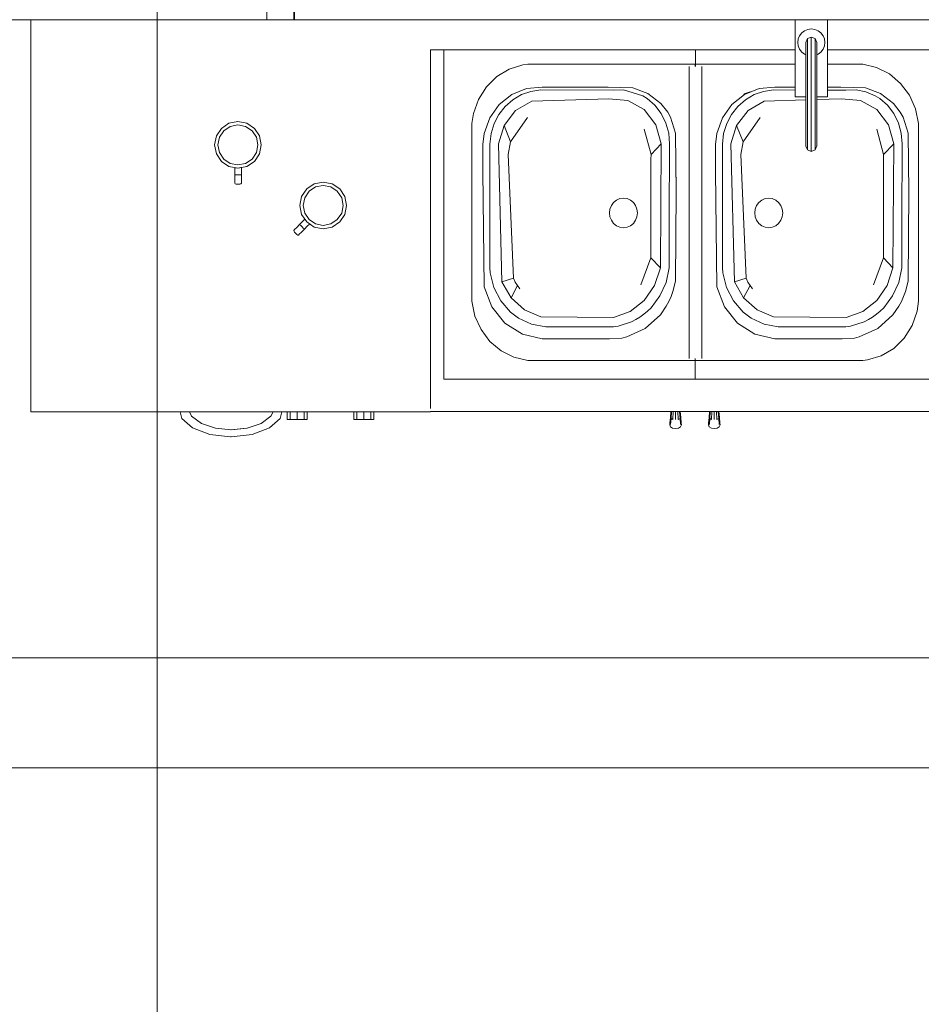
# Model space of a CAD drawing. Units: feet. Extents: x -297 to 770, y -228 to 625.
# Tile 11 of 14: x 680 to 716, y 194 to 233. Entities that reach past the tile are written whole.
import ezdxf

# ---------------------------------------------------------------- set-up
doc = ezdxf.new("R2010")
doc.units = ezdxf.units.FT
doc.header["$MEASUREMENT"] = 0
for name, color, linetype, lineweight in [('A-ANNO-DIMS', 2, 'Continuous', 18), ('A-EQPM', 8, 'Continuous', 13), ('A-FLOR-CASE', 8, 'Continuous', 18), ('A-FLOR-FIXT', 8, 'Continuous', 18), ('A-WALL', 7, 'Continuous', 35), ('doors', 30, 'Continuous', 18)]:
    doc.layers.add(name, color=color, linetype=linetype, lineweight=lineweight)
doc.styles.get("Standard").update_dxf_attribs({"font": 'arial.ttf'})
doc.dimstyles.get("Standard").update_dxf_attribs({"dimtxt": 3, "dimasz": 2, "dimexe": 0.18, "dimexo": 0.0625, "dimgap": 0.09, "dimtad": 1, "dimtoh": 1, "dimdec": 1, "dimzin": 0, "dimdsep": 46, "dimlunit": 3, "dimtxsty": 'Standard', "dimcen": 0, "dimclre": 256, "dimadec": 0, "dimazin": 0, "dimtfac": 1, "dimtdec": 1, "dimtofl": 0, "dimtmove": 0, "dimatfit": 3, "dimfxl": 1, "dimtolj": 1, "dimtzin": 0, "dimlwe": -1, "dimarcsym": 0})

# ---------------------------------------------------------------- blocks, each defined once
blk = doc.blocks.new('*U6')
for p, q in [((0, 0), (0, -6)), ((40, 0), (40, -6))]:
    blk.add_line(p, q)
blk.add_lwpolyline([(0, 0), (0, 40), (1.75, 40), (1.75, 0)], close=True)
blk.add_arc((0, 0), 40, 0, 90)
blk = doc.blocks.new('*D54')
at = {"layer": 'A-ANNO-DIMS', "transparency": 16777216}
for p, q in [((733.096, 233.463), (354.525, 233.463)), ((733.093, 203.463), (354.525, 203.463))]:
    blk.add_line(p, q, dxfattribs=at)
at = {"layer": 'A-ANNO-DIMS', "color": 0, "lineweight": -2, "transparency": 16777216}
blk.add_line((354.705, 205.463), (354.705, 231.463), dxfattribs=at)
at = {"layer": 'A-ANNO-DIMS', "color": 0, "transparency": 16777216}
for points in [[(354.372, 231.463), (355.039, 231.463), (354.705, 233.463)], [(354.372, 205.463), (355.039, 205.463), (354.705, 203.463)]]:
    blk.add_solid(points, dxfattribs=at)
at = {"layer": 'Defpoints', "color": 0, "transparency": 16777216}
for p in [(354.705, 233.463), (733.158, 233.463), (733.155, 203.463)]:
    blk.add_point(p, dxfattribs=at)
at = {"layer": 'A-ANNO-DIMS', "color": 0, "transparency": 16777216, "insert": (353.083, 218.463), "char_height": 3, "attachment_point": 5, "rotation": 90}
blk.add_mtext('\\A1;30', dxfattribs=at)
blk = doc.blocks.new('*D68')
at = {"layer": 'A-ANNO-DIMS', "transparency": 16777216}
for p, q in [((685.155, 306.9), (685.155, -227.667)), ((721.155, 306.9), (721.155, -227.667))]:
    blk.add_line(p, q, dxfattribs=at)
at = {"layer": 'A-ANNO-DIMS', "color": 0, "lineweight": -2, "transparency": 16777216}
blk.add_line((687.155, -227.487), (719.155, -227.487), dxfattribs=at)
at = {"layer": 'A-ANNO-DIMS', "color": 0, "transparency": 16777216}
for points in [[(687.155, -227.154), (687.155, -227.821), (685.155, -227.487)], [(719.155, -227.154), (719.155, -227.821), (721.155, -227.487)]]:
    blk.add_solid(points, dxfattribs=at)
at = {"layer": 'Defpoints', "color": 0, "transparency": 16777216}
for p in [(685.155, 306.963), (721.155, 306.963), (721.155, -227.487)]:
    blk.add_point(p, dxfattribs=at)
at = {"layer": 'A-ANNO-DIMS', "color": 0, "transparency": 16777216, "insert": (703.155, -225.865), "char_height": 3, "attachment_point": 5}
blk.add_mtext('\\A1;36', dxfattribs=at)
blk = doc.blocks.new('*D75')
at = {"layer": 'A-ANNO-DIMS', "transparency": 16777216}
for p, q in [((471.753, 264.961), (769.785, 264.961)), ((471.753, 207.869), (769.785, 207.869))]:
    blk.add_line(p, q, dxfattribs=at)
at = {"layer": 'A-ANNO-DIMS', "color": 0, "lineweight": -2, "transparency": 16777216}
blk.add_line((769.605, 209.869), (769.605, 262.961), dxfattribs=at)
at = {"layer": 'A-ANNO-DIMS', "color": 0, "transparency": 16777216}
for points in [[(769.272, 262.961), (769.939, 262.961), (769.605, 264.961)], [(769.272, 209.869), (769.939, 209.869), (769.605, 207.869)]]:
    blk.add_solid(points, dxfattribs=at)
at = {"layer": 'Defpoints', "color": 0, "transparency": 16777216}
for p in [(471.691, 264.961), (769.605, 264.961), (471.691, 207.869)]:
    blk.add_point(p, dxfattribs=at)
at = {"layer": 'A-ANNO-DIMS', "color": 0, "transparency": 16777216, "insert": (767.984, 236.415), "char_height": 3, "attachment_point": 5, "rotation": 90}
blk.add_mtext('\\A1;57.09', dxfattribs=at)

msp = doc.modelspace()

# ---------------------------------------------------------------- linework, layer by layer
at = {"layer": 'A-EQPM'}
for p, q in [((687.735, 229.103), (687.533, 228.8)), ((688.039, 229.306), (687.735, 229.103)), ((688.09, 229.183), (687.83, 229.009)), ((688.397, 229.378), (688.039, 229.306)), ((688.397, 229.244), (688.09, 229.183)), ((688.755, 229.306), (688.397, 229.378)), ((688.704, 229.183), (688.397, 229.244)), ((688.964, 229.009), (688.704, 229.183)), ((689.059, 229.103), (688.755, 229.306)), ((689.262, 228.8), (689.059, 229.103)), ((687.533, 228.8), (687.461, 228.442)), ((687.656, 228.749), (687.595, 228.442)), ((687.83, 229.009), (687.656, 228.749)), ((689.138, 228.749), (688.964, 229.009)), ((689.199, 228.442), (689.138, 228.749)), ((689.333, 228.442), (689.262, 228.8)), ((687.461, 228.442), (687.533, 228.083)), ((687.595, 228.442), (687.656, 228.135)), ((689.138, 228.135), (689.199, 228.442)), ((689.262, 228.083), (689.333, 228.442)), ((687.533, 228.083), (687.735, 227.78)), ((687.656, 228.135), (687.83, 227.874)), ((687.83, 227.874), (688.09, 227.7)), ((688.704, 227.7), (688.964, 227.874)), ((688.964, 227.874), (689.138, 228.135)), ((689.059, 227.78), (689.262, 228.083)), ((687.735, 227.78), (688.039, 227.577)), ((688.039, 227.577), (688.397, 227.505)), ((688.09, 227.7), (688.397, 227.639)), ((688.268, 226.9), (688.268, 227.531)), ((688.274, 227.53), (688.275, 227.53)), ((688.275, 227.53), (688.277, 227.529)), ((688.334, 227.518), (688.299, 227.525)), ((688.397, 227.505), (688.334, 227.518)), ((688.397, 227.639), (688.704, 227.7)), ((688.397, 227.505), (688.755, 227.577)), ((688.436, 227.513), (688.517, 227.529)), ((688.468, 227.52), (688.525, 227.531)), ((688.525, 227.531), (688.517, 227.529)), ((688.525, 227.531), (688.535, 227.533)), ((688.535, 227.533), (688.535, 227.401)), ((688.755, 227.577), (689.059, 227.78)), ((688.268, 227.234), (688.285, 227.234)), ((688.285, 227.234), (688.517, 227.234)), ((688.535, 227.234), (688.517, 227.234)), ((688.535, 227.401), (688.535, 227.234)), ((688.535, 227.067), (688.535, 227.234)), ((688.285, 226.883), (688.268, 226.9)), ((688.334, 226.871), (688.285, 226.883)), ((688.401, 226.866), (688.334, 226.871)), ((688.468, 226.871), (688.401, 226.866)), ((688.517, 226.883), (688.468, 226.871)), ((688.535, 226.9), (688.517, 226.883)), ((688.535, 227.067), (688.535, 226.9)), ((691.461, 226.877), (691.158, 226.674)), ((691.512, 226.753), (691.252, 226.579)), ((691.819, 226.948), (691.461, 226.877)), ((691.819, 226.814), (691.512, 226.753)), ((692.177, 226.877), (691.819, 226.948)), ((692.126, 226.753), (691.819, 226.814)), ((692.386, 226.579), (692.126, 226.753)), ((692.481, 226.674), (692.177, 226.877)), ((690.955, 226.37), (690.883, 226.012)), ((691.158, 226.674), (690.955, 226.37)), ((691.078, 226.319), (691.017, 226.012)), ((691.252, 226.579), (691.078, 226.319)), ((692.56, 226.319), (692.386, 226.579)), ((692.684, 226.37), (692.481, 226.674)), ((692.621, 226.012), (692.56, 226.319)), ((692.755, 226.012), (692.684, 226.37)), ((690.883, 226.012), (690.955, 225.654)), ((691.017, 226.012), (691.078, 225.705)), ((692.56, 225.705), (692.621, 226.012)), ((692.684, 225.654), (692.755, 226.012)), ((690.955, 225.654), (691.158, 225.35)), ((691.078, 225.705), (691.252, 225.445)), ((692.386, 225.445), (692.56, 225.705)), ((692.481, 225.35), (692.684, 225.654)), ((690.756, 225.131), (690.669, 225.045)), ((690.756, 225.131), (690.874, 225.25)), ((690.874, 225.25), (690.992, 225.368)), ((690.874, 225.25), (690.887, 225.237)), ((690.887, 225.237), (690.921, 225.202)), ((690.921, 225.202), (690.969, 225.155)), ((690.969, 225.155), (691.016, 225.108)), ((690.992, 225.368), (691.084, 225.46)), ((691.016, 225.108), (691.05, 225.073)), ((691.063, 225.061), (691.181, 225.179)), ((691.089, 225.452), (691.094, 225.445)), ((691.094, 225.445), (691.114, 225.416)), ((691.158, 225.35), (691.461, 225.147)), ((691.181, 225.179), (691.268, 225.265)), ((691.189, 225.329), (691.218, 225.31)), ((691.218, 225.31), (691.257, 225.283)), ((691.252, 225.445), (691.512, 225.271)), ((691.268, 225.265), (691.274, 225.272)), ((691.274, 225.272), (691.273, 225.273)), ((691.461, 225.147), (691.819, 225.076)), ((691.512, 225.271), (691.819, 225.21)), ((691.819, 225.21), (692.126, 225.271)), ((691.819, 225.076), (692.177, 225.147)), ((692.126, 225.271), (692.386, 225.445)), ((692.177, 225.147), (692.481, 225.35)), ((690.669, 225.045), (690.638, 225.013)), ((690.638, 225.013), (690.638, 224.989)), ((690.638, 224.989), (690.664, 224.946)), ((690.664, 224.946), (690.709, 224.895)), ((690.709, 224.895), (690.759, 224.851)), ((690.759, 224.851), (690.802, 224.825)), ((690.802, 224.825), (690.827, 224.824)), ((690.827, 224.824), (690.858, 224.856)), ((690.858, 224.856), (690.945, 224.942)), ((690.945, 224.942), (691.063, 225.061)), ((691.063, 225.061), (691.05, 225.073))]:
    msp.add_line(p, q, dxfattribs=at)
at = {"layer": 'A-FLOR-CASE'}
for p, q in [((680.083, 217.736), (680.083, 233.463)), ((680.083, 233.463), (733.158, 233.463)), ((696.125, 217.869), (696.125, 232.254)), ((680.083, 217.736), (680.083, 217.87)), ((696.125, 217.736), (680.083, 217.736)), ((686.075, 217.736), (686.143, 217.472)), ((686.449, 217.736), (686.54, 217.555)), ((689.724, 217.555), (689.815, 217.736)), ((690.094, 217.472), (690.162, 217.736)), ((690.377, 217.43), (690.377, 217.736)), ((690.494, 217.736), (690.494, 217.43)), ((690.778, 217.43), (690.778, 217.736)), ((691.061, 217.43), (691.061, 217.736)), ((691.179, 217.43), (691.179, 217.736)), ((693.051, 217.43), (693.051, 217.736)), ((693.168, 217.736), (693.168, 217.43)), ((693.452, 217.43), (693.452, 217.736)), ((693.735, 217.43), (693.735, 217.736)), ((693.853, 217.43), (693.853, 217.736)), ((696.125, 217.748), (717.37, 217.748)), ((705.747, 217.512), (705.769, 217.748)), ((705.775, 217.467), (705.796, 217.748)), ((705.865, 217.748), (705.852, 217.434)), ((705.956, 217.422), (705.956, 217.748)), ((706.048, 217.748), (706.061, 217.434)), ((706.137, 217.467), (706.116, 217.748)), ((706.143, 217.748), (706.165, 217.512)), ((707.299, 217.512), (707.321, 217.748)), ((707.327, 217.467), (707.348, 217.748)), ((707.416, 217.748), (707.403, 217.434)), ((707.508, 217.422), (707.508, 217.748)), ((707.599, 217.748), (707.612, 217.434)), ((707.689, 217.467), (707.668, 217.748)), ((707.695, 217.748), (707.717, 217.512)), ((686.143, 217.472), (686.578, 217.087)), ((686.54, 217.555), (686.939, 217.267)), ((686.939, 217.267), (687.494, 217.08)), ((688.77, 217.08), (689.325, 217.267)), ((689.325, 217.267), (689.724, 217.555)), ((689.659, 217.087), (690.094, 217.472)), ((690.494, 217.43), (690.377, 217.43)), ((690.494, 217.43), (690.778, 217.43)), ((690.778, 217.43), (691.061, 217.43)), ((691.061, 217.43), (691.179, 217.43)), ((693.168, 217.43), (693.051, 217.43)), ((693.168, 217.43), (693.452, 217.43)), ((693.452, 217.43), (693.735, 217.43)), ((693.735, 217.43), (693.853, 217.43)), ((705.722, 217.208), (705.728, 217.287)), ((705.753, 217.136), (705.722, 217.208)), ((705.728, 217.287), (705.747, 217.512)), ((705.747, 217.512), (705.775, 217.467)), ((705.775, 217.467), (705.759, 217.223)), ((705.852, 217.434), (705.775, 217.467)), ((706.061, 217.434), (706.137, 217.467)), ((706.165, 217.512), (706.137, 217.467)), ((706.137, 217.467), (706.153, 217.223)), ((706.19, 217.208), (706.159, 217.136)), ((706.165, 217.512), (706.184, 217.287)), ((706.184, 217.287), (706.19, 217.208)), ((707.274, 217.208), (707.28, 217.287)), ((707.305, 217.136), (707.274, 217.208)), ((707.28, 217.287), (707.299, 217.512)), ((707.299, 217.512), (707.327, 217.467)), ((707.327, 217.467), (707.311, 217.223)), ((707.403, 217.434), (707.327, 217.467)), ((707.612, 217.434), (707.689, 217.467)), ((707.717, 217.512), (707.689, 217.467)), ((707.689, 217.467), (707.705, 217.223)), ((707.742, 217.208), (707.71, 217.136)), ((707.717, 217.512), (707.735, 217.287)), ((707.735, 217.287), (707.742, 217.208)), ((686.578, 217.087), (687.271, 216.824)), ((687.271, 216.824), (688.105, 216.73)), ((687.494, 217.08), (688.132, 217.016)), ((688.119, 217.017), (688.743, 217.08)), ((688.132, 217.016), (688.77, 217.08)), ((688.132, 216.73), (688.966, 216.824)), ((688.966, 216.824), (689.659, 217.087)), ((705.839, 217.084), (705.753, 217.136)), ((705.956, 217.065), (705.839, 217.084)), ((706.073, 217.084), (705.956, 217.065)), ((706.159, 217.136), (706.073, 217.084)), ((707.391, 217.084), (707.305, 217.136)), ((707.508, 217.065), (707.391, 217.084)), ((707.625, 217.084), (707.508, 217.065)), ((707.71, 217.136), (707.625, 217.084)), ((688.105, 216.73), (688.119, 216.732))]:
    msp.add_line(p, q, dxfattribs=at)
at = {"layer": 'A-FLOR-FIXT'}
for p, q in [((710.749, 230.375), (710.749, 233.463)), ((712.053, 230.375), (712.053, 233.463)), ((711.129, 233.02), (711.017, 232.934)), ((711.26, 233.074), (711.129, 233.02)), ((711.401, 233.093), (711.26, 233.074)), ((711.541, 233.074), (711.401, 233.093)), ((711.673, 233.02), (711.541, 233.074)), ((711.785, 232.934), (711.673, 233.02)), ((710.876, 232.69), (710.857, 232.549)), ((710.93, 232.821), (710.876, 232.69)), ((711.017, 232.934), (710.93, 232.821)), ((711.183, 232.549), (711.247, 232.703)), ((711.183, 232.549), (711.216, 232.629)), ((711.401, 232.767), (711.247, 232.703)), ((711.247, 232.703), (711.323, 232.735)), ((711.247, 232.703), (711.247, 232.121)), ((711.554, 232.703), (711.401, 232.767)), ((711.401, 232.767), (711.481, 232.733)), ((711.401, 232.168), (711.401, 232.767)), ((711.618, 232.549), (711.554, 232.703)), ((711.554, 232.703), (711.581, 232.639)), ((711.554, 232.121), (711.554, 232.703)), ((711.871, 232.821), (711.785, 232.934)), ((711.926, 232.69), (711.871, 232.821)), ((711.944, 232.549), (711.926, 232.69)), ((710.749, 232.254), (696.125, 232.254)), ((696.662, 219.047), (696.662, 232.254)), ((706.751, 231.676), (706.751, 232.254)), ((710.857, 232.549), (710.876, 232.409)), ((710.876, 232.409), (710.93, 232.277)), ((710.93, 232.277), (711.017, 232.165)), ((711.183, 232.007), (711.183, 232.549)), ((711.618, 232.007), (711.618, 232.549)), ((711.785, 232.165), (711.871, 232.277)), ((711.871, 232.277), (711.926, 232.409)), ((711.926, 232.409), (711.944, 232.549)), ((712.053, 232.254), (717.503, 232.254)), ((711.017, 232.165), (711.129, 232.079)), ((711.129, 232.079), (711.183, 232.056)), ((711.184, 231.724), (711.183, 232.007)), ((711.247, 232.121), (711.247, 231.817)), ((711.247, 231.817), (711.247, 231.467)), ((711.401, 231.855), (711.401, 232.168)), ((711.401, 231.495), (711.401, 231.855)), ((711.555, 231.817), (711.554, 232.121)), ((711.555, 231.467), (711.555, 231.817)), ((711.618, 232.056), (711.673, 232.079)), ((711.619, 231.724), (711.618, 232.007)), ((711.673, 232.079), (711.785, 232.165)), ((698.784, 231.185), (699.284, 231.484)), ((699.284, 231.484), (699.834, 231.651)), ((699.834, 231.651), (700.025, 231.676)), ((700.025, 231.676), (706.751, 231.676)), ((706.499, 219.877), (706.499, 231.589)), ((706.74, 231.676), (707.085, 231.676)), ((706.74, 231.589), (706.74, 231.676)), ((706.751, 231.676), (706.751, 231.589)), ((707.003, 219.877), (707.003, 231.589)), ((707.085, 231.676), (710.749, 231.676)), ((711.184, 231.398), (711.184, 231.724)), ((711.247, 231.467), (711.248, 231.083)), ((711.401, 231.101), (711.401, 231.495)), ((711.555, 231.083), (711.555, 231.467)), ((711.619, 231.041), (711.619, 231.724)), ((713.466, 231.676), (712.053, 231.676)), ((714.023, 231.546), (713.466, 231.676)), ((714.538, 231.285), (714.023, 231.546)), ((698.364, 230.773), (698.784, 231.185)), ((711.184, 231.041), (711.184, 231.398)), ((711.184, 230.664), (711.184, 231.041)), ((711.248, 231.083), (711.248, 230.679)), ((711.401, 230.685), (711.401, 231.101)), ((711.555, 230.679), (711.555, 231.083)), ((711.619, 230.665), (711.619, 231.041)), ((714.984, 230.909), (714.538, 231.285)), ((698.045, 230.268), (698.364, 230.773)), ((699.975, 230.698), (699.384, 230.461)), ((700.605, 230.751), (699.975, 230.698)), ((700.545, 230.643), (700.152, 230.589)), ((703.459, 230.64), (700.545, 230.643)), ((703.256, 230.751), (700.605, 230.751)), ((704.241, 230.731), (703.256, 230.751)), ((703.864, 230.648), (703.459, 230.64)), ((704.636, 230.411), (703.864, 230.648)), ((704.849, 230.509), (704.241, 230.731)), ((709.308, 230.698), (708.717, 230.461)), ((709.937, 230.751), (709.308, 230.698)), ((709.878, 230.643), (709.484, 230.589)), ((710.749, 230.642), (709.878, 230.643)), ((710.749, 230.751), (709.937, 230.751)), ((711.184, 230.281), (711.184, 230.664)), ((711.248, 230.679), (711.248, 230.267)), ((711.402, 230.261), (711.401, 230.685)), ((711.555, 230.267), (711.555, 230.679)), ((711.619, 230.281), (711.619, 230.665)), ((712.588, 230.751), (712.053, 230.751)), ((712.791, 230.64), (712.053, 230.64)), ((713.574, 230.731), (712.588, 230.751)), ((713.196, 230.648), (712.791, 230.64)), ((713.593, 230.571), (713.196, 230.648)), ((714.182, 230.509), (713.574, 230.731)), ((715.339, 230.435), (714.984, 230.909)), ((697.845, 229.7), (698.045, 230.268)), ((699.384, 230.461), (698.879, 230.058)), ((699.425, 230.255), (699.12, 229.987)), ((699.775, 230.459), (699.425, 230.255)), ((700.152, 230.589), (699.775, 230.459)), ((700.183, 230.193), (703.275, 230.292)), ((703.275, 230.292), (704.038, 230.228)), ((704.811, 230.301), (704.636, 230.411)), ((705.124, 230.031), (704.811, 230.301)), ((705.368, 230.104), (704.849, 230.509)), ((708.717, 230.461), (708.212, 230.058)), ((708.758, 230.255), (708.453, 229.987)), ((708.685, 230.435), (708.713, 230.486)), ((708.713, 230.486), (708.702, 230.449)), ((708.713, 230.486), (708.746, 230.498)), ((708.746, 230.498), (708.87, 230.544)), ((709.107, 230.459), (708.758, 230.255)), ((708.87, 230.544), (708.905, 230.552)), ((709.011, 230.579), (708.905, 230.552)), ((708.905, 230.552), (708.973, 230.569)), ((708.973, 230.569), (709.011, 230.579)), ((709.484, 230.589), (709.107, 230.459)), ((709.516, 230.193), (711.184, 230.246)), ((710.771, 230.375), (710.749, 230.375)), ((710.836, 230.375), (710.771, 230.375)), ((710.94, 230.375), (710.836, 230.375)), ((711.075, 230.375), (710.94, 230.375)), ((711.184, 230.375), (711.075, 230.375)), ((711.184, 229.905), (711.184, 230.281)), ((711.248, 230.267), (711.248, 229.863)), ((711.402, 229.845), (711.402, 230.261)), ((711.555, 229.863), (711.555, 230.267)), ((711.619, 230.375), (712.031, 230.375)), ((711.619, 230.26), (712.608, 230.292)), ((711.619, 229.905), (711.619, 230.281)), ((712.031, 230.375), (712.053, 230.375)), ((712.608, 230.292), (713.37, 230.228)), ((713.969, 230.411), (713.593, 230.571)), ((714.144, 230.301), (713.969, 230.411)), ((714.457, 230.031), (714.144, 230.301)), ((714.7, 230.104), (714.182, 230.509)), ((715.585, 229.889), (715.339, 230.435)), ((698.879, 230.058), (698.499, 229.523)), ((699.12, 229.987), (698.867, 229.663)), ((699.54, 229.818), (700.183, 230.193)), ((704.038, 230.228), (704.699, 229.86)), ((704.699, 229.86), (705.17, 229.248)), ((705.379, 229.699), (705.124, 230.031)), ((705.639, 229.752), (705.368, 230.104)), ((708.212, 230.058), (707.832, 229.523)), ((708.453, 229.987), (708.2, 229.663)), ((708.873, 229.818), (709.516, 230.193)), ((711.185, 229.547), (711.184, 229.905)), ((711.248, 229.863), (711.248, 229.479)), ((711.402, 229.451), (711.402, 229.845)), ((711.556, 229.479), (711.555, 229.863)), ((711.619, 229.222), (711.619, 229.905)), ((713.37, 230.228), (714.032, 229.86)), ((714.032, 229.86), (714.503, 229.248)), ((714.712, 229.699), (714.457, 230.031)), ((714.972, 229.752), (714.7, 230.104)), ((715.708, 229.299), (715.585, 229.889)), ((697.783, 229.299), (697.845, 229.7)), ((698.499, 229.523), (698.276, 228.896)), ((698.867, 229.663), (698.675, 229.293)), ((699.073, 229.22), (699.54, 229.818)), ((699.329, 228.568), (700.014, 229.535)), ((705.568, 229.318), (705.379, 229.699)), ((705.749, 229.555), (705.639, 229.752)), ((705.959, 228.91), (705.749, 229.555)), ((707.832, 229.523), (707.608, 228.896)), ((708.2, 229.663), (708.008, 229.293)), ((708.406, 229.22), (708.873, 229.818)), ((708.662, 228.568), (709.347, 229.535)), ((711.185, 228.938), (711.185, 229.547)), ((711.248, 229.479), (711.248, 228.825)), ((711.402, 228.778), (711.402, 229.451)), ((711.556, 228.825), (711.556, 229.479)), ((714.901, 229.318), (714.712, 229.699)), ((715.082, 229.555), (714.972, 229.752)), ((715.291, 228.91), (715.082, 229.555)), ((697.783, 222.167), (697.783, 229.299)), ((698.675, 229.293), (698.552, 228.893)), ((698.846, 228.482), (699.073, 229.22)), ((699.073, 229.22), (699.329, 228.568)), ((704.971, 228.053), (704.693, 229.071)), ((705.17, 229.248), (705.378, 228.489)), ((705.68, 228.906), (705.568, 229.318)), ((708.008, 229.293), (707.885, 228.893)), ((708.179, 228.482), (708.406, 229.22)), ((708.406, 229.22), (708.662, 228.568)), ((711.62, 228.939), (711.619, 229.222)), ((714.304, 228.053), (714.026, 229.071)), ((714.503, 229.248), (714.711, 228.489)), ((715.013, 228.906), (714.901, 229.318)), ((715.708, 222.167), (715.708, 229.299)), ((698.276, 228.896), (698.222, 228.453)), ((698.552, 228.893), (698.502, 228.476)), ((705.713, 228.48), (705.68, 228.906)), ((705.978, 226.546), (705.959, 228.91)), ((707.608, 228.896), (707.555, 228.453)), ((707.885, 228.893), (707.835, 228.476)), ((711.185, 228.708), (711.185, 228.938)), ((711.185, 228.396), (711.185, 228.708)), ((711.248, 228.825), (711.249, 228.577)), ((711.402, 228.523), (711.402, 228.778)), ((711.556, 228.577), (711.556, 228.825)), ((711.62, 228.397), (711.62, 228.939)), ((715.045, 228.48), (715.013, 228.906)), ((715.31, 226.546), (715.291, 228.91)), ((698.222, 228.453), (698.225, 228.228)), ((698.502, 228.476), (698.505, 223.515)), ((698.846, 228.482), (698.987, 222.954)), ((699.329, 228.568), (699.243, 228.05)), ((705.378, 228.489), (704.971, 228.053)), ((705.345, 223.504), (705.378, 228.489)), ((705.698, 225.409), (705.713, 228.48)), ((707.555, 228.453), (707.558, 228.228)), ((707.835, 228.476), (707.837, 223.515)), ((708.179, 228.482), (708.32, 222.954)), ((708.662, 228.568), (708.576, 228.05)), ((711.249, 228.243), (711.185, 228.396)), ((711.249, 228.577), (711.249, 228.243)), ((711.402, 228.179), (711.402, 228.523)), ((711.556, 228.243), (711.556, 228.577)), ((711.556, 228.243), (711.62, 228.397)), ((714.711, 228.489), (714.304, 228.053)), ((714.677, 223.504), (714.711, 228.489)), ((715.031, 225.409), (715.045, 228.48)), ((698.225, 228.228), (698.225, 227.387)), ((699.243, 228.05), (699.449, 223.09)), ((704.959, 227.874), (704.971, 228.053)), ((704.959, 223.908), (704.959, 227.874)), ((707.558, 228.228), (707.558, 227.387)), ((708.576, 228.05), (708.782, 223.09)), ((711.249, 228.243), (711.402, 228.179)), ((711.402, 228.179), (711.556, 228.243)), ((714.292, 227.874), (714.304, 228.053)), ((714.292, 223.908), (714.292, 227.874)), ((698.225, 227.387), (698.281, 222.752)), ((705.973, 227.174), (705.999, 227.114)), ((707.558, 227.387), (707.614, 222.752)), ((703.72, 226.288), (703.585, 226.229)), ((703.865, 226.308), (703.72, 226.288)), ((704.011, 226.288), (703.865, 226.308)), ((704.146, 226.229), (704.011, 226.288)), ((705.949, 222.97), (705.978, 226.546)), ((709.547, 226.288), (709.411, 226.229)), ((709.692, 226.308), (709.547, 226.288)), ((709.837, 226.288), (709.692, 226.308)), ((709.973, 226.229), (709.837, 226.288)), ((715.281, 222.97), (715.31, 226.546)), ((703.379, 226.011), (703.323, 225.867)), ((703.468, 226.134), (703.379, 226.011)), ((703.585, 226.229), (703.468, 226.134)), ((704.262, 226.134), (704.146, 226.229)), ((704.351, 226.011), (704.262, 226.134)), ((704.408, 225.867), (704.351, 226.011)), ((709.206, 226.011), (709.15, 225.867)), ((709.295, 226.134), (709.206, 226.011)), ((709.411, 226.229), (709.295, 226.134)), ((710.089, 226.134), (709.973, 226.229)), ((710.178, 226.011), (710.089, 226.134)), ((710.234, 225.867), (710.178, 226.011)), ((703.323, 225.867), (703.304, 225.713)), ((703.304, 225.713), (703.323, 225.559)), ((703.323, 225.559), (703.379, 225.416)), ((704.351, 225.416), (704.408, 225.559)), ((704.427, 225.713), (704.408, 225.867)), ((704.408, 225.559), (704.427, 225.713)), ((709.15, 225.867), (709.131, 225.713)), ((709.131, 225.713), (709.15, 225.559)), ((709.15, 225.559), (709.206, 225.416)), ((710.178, 225.416), (710.234, 225.559)), ((710.253, 225.713), (710.234, 225.867)), ((710.234, 225.559), (710.253, 225.713)), ((703.379, 225.416), (703.468, 225.292)), ((703.468, 225.292), (703.585, 225.198)), ((703.585, 225.198), (703.72, 225.138)), ((703.72, 225.138), (703.865, 225.118)), ((703.865, 225.118), (704.011, 225.138)), ((704.011, 225.138), (704.146, 225.198)), ((704.146, 225.198), (704.262, 225.292)), ((704.262, 225.292), (704.351, 225.416)), ((705.698, 223.515), (705.698, 225.409)), ((709.206, 225.416), (709.295, 225.292)), ((709.295, 225.292), (709.411, 225.198)), ((709.411, 225.198), (709.547, 225.138)), ((709.547, 225.138), (709.692, 225.118)), ((709.692, 225.118), (709.837, 225.138)), ((709.837, 225.138), (709.973, 225.198)), ((709.973, 225.198), (710.089, 225.292)), ((710.089, 225.292), (710.178, 225.416)), ((715.031, 223.515), (715.031, 225.409)), ((704.959, 223.908), (704.561, 222.822)), ((705.345, 223.504), (704.959, 223.908)), ((714.292, 223.908), (713.894, 222.822)), ((714.677, 223.504), (714.292, 223.908)), ((698.505, 223.515), (698.523, 223.311)), ((698.523, 223.311), (698.67, 222.721)), ((705.115, 222.801), (705.345, 223.504)), ((705.574, 222.926), (705.698, 223.515)), ((707.837, 223.515), (707.856, 223.311)), ((707.856, 223.311), (708.003, 222.721)), ((714.448, 222.801), (714.677, 223.504)), ((714.907, 222.926), (715.031, 223.515)), ((698.281, 222.752), (698.583, 221.95)), ((699.449, 223.09), (698.987, 222.954)), ((698.987, 222.954), (699.354, 222.308)), ((699.354, 222.308), (699.615, 222.798)), ((699.527, 222.94), (699.449, 223.09)), ((699.615, 222.798), (699.527, 222.94)), ((699.615, 222.798), (699.714, 222.663)), ((704.699, 222.201), (705.115, 222.801)), ((705.328, 222.381), (705.574, 222.926)), ((705.846, 222.556), (705.949, 222.97)), ((707.614, 222.752), (707.916, 221.95)), ((708.782, 223.09), (708.32, 222.954)), ((708.32, 222.954), (708.687, 222.308)), ((708.687, 222.308), (708.948, 222.798)), ((708.86, 222.94), (708.782, 223.09)), ((708.948, 222.798), (708.86, 222.94)), ((708.948, 222.798), (709.047, 222.663)), ((714.031, 222.201), (714.448, 222.801)), ((714.661, 222.381), (714.907, 222.926)), ((715.178, 222.556), (715.281, 222.97)), ((698.67, 222.721), (698.948, 222.184)), ((704.974, 221.909), (705.328, 222.381)), ((705.685, 222.164), (705.773, 222.357)), ((705.773, 222.357), (705.846, 222.556)), ((708.003, 222.721), (708.28, 222.184)), ((714.306, 221.909), (714.661, 222.381)), ((715.018, 222.164), (715.105, 222.357)), ((715.105, 222.357), (715.178, 222.556)), ((697.906, 221.577), (697.783, 222.167)), ((698.583, 221.95), (699.11, 221.292)), ((698.948, 222.184), (699.338, 221.735)), ((699.354, 222.308), (699.896, 221.82)), ((704.132, 221.759), (704.699, 222.201)), ((705.345, 221.632), (705.585, 221.977)), ((705.585, 221.977), (705.685, 222.164)), ((707.916, 221.95), (708.443, 221.292)), ((708.28, 222.184), (708.671, 221.735)), ((708.687, 222.308), (709.228, 221.82)), ((713.465, 221.759), (714.031, 222.201)), ((714.677, 221.632), (714.917, 221.977)), ((714.917, 221.977), (715.018, 222.164)), ((715.646, 221.767), (715.708, 222.167)), ((698.152, 221.031), (697.906, 221.577)), ((699.338, 221.735), (699.651, 221.497)), ((699.896, 221.82), (700.556, 221.541)), ((703.469, 221.516), (704.132, 221.759)), ((704.528, 221.532), (704.686, 221.646)), ((704.686, 221.646), (704.834, 221.772)), ((704.734, 221.076), (705.345, 221.632)), ((704.834, 221.772), (704.974, 221.909)), ((705.467, 221.809), (705.469, 221.811)), ((708.671, 221.735), (708.983, 221.497)), ((709.228, 221.82), (709.888, 221.541)), ((712.802, 221.516), (713.465, 221.759)), ((713.861, 221.532), (714.018, 221.646)), ((714.018, 221.646), (714.167, 221.772)), ((714.067, 221.076), (714.677, 221.632)), ((714.167, 221.772), (714.306, 221.909)), ((715.446, 221.198), (715.646, 221.767)), ((699.11, 221.292), (699.809, 220.845)), ((699.651, 221.497), (700.177, 221.248)), ((700.177, 221.248), (700.745, 221.14)), ((700.556, 221.541), (703.469, 221.516)), ((703.459, 221.14), (703.647, 221.169)), ((703.647, 221.169), (704.191, 221.345)), ((704.191, 221.345), (704.363, 221.432)), ((704.363, 221.432), (704.528, 221.532)), ((708.443, 221.292), (709.142, 220.845)), ((708.983, 221.497), (709.51, 221.248)), ((709.51, 221.248), (710.077, 221.14)), ((709.888, 221.541), (712.802, 221.516)), ((712.791, 221.14), (712.98, 221.169)), ((712.98, 221.169), (713.524, 221.345)), ((713.524, 221.345), (713.695, 221.432)), ((713.695, 221.432), (713.861, 221.532)), ((715.126, 220.693), (715.446, 221.198)), ((698.507, 220.557), (698.152, 221.031)), ((699.809, 220.845), (700.605, 220.659)), ((700.745, 221.14), (703.459, 221.14)), ((703.996, 220.737), (704.734, 221.076)), ((709.142, 220.845), (709.937, 220.659)), ((710.077, 221.14), (712.791, 221.14)), ((713.328, 220.737), (714.067, 221.076)), ((698.953, 220.181), (698.507, 220.557)), ((700.605, 220.659), (703.309, 220.659)), ((703.309, 220.659), (703.799, 220.69)), ((703.799, 220.69), (703.996, 220.737)), ((709.937, 220.659), (712.642, 220.659)), ((712.642, 220.659), (713.131, 220.69)), ((713.131, 220.69), (713.328, 220.737)), ((714.706, 220.281), (715.126, 220.693)), ((699.468, 219.921), (698.953, 220.181)), ((713.656, 219.815), (714.206, 219.982)), ((714.206, 219.982), (714.706, 220.281)), ((700.025, 219.79), (699.468, 219.921)), ((706.406, 219.79), (700.025, 219.79)), ((706.751, 219.79), (706.406, 219.79)), ((706.74, 219.047), (706.74, 219.877)), ((706.74, 219.79), (713.466, 219.79)), ((713.466, 219.79), (713.656, 219.815)), ((706.751, 219.047), (696.662, 219.047)), ((696.662, 219.047), (707.003, 219.047)), ((706.499, 219.047), (716.841, 219.047)), ((716.841, 219.047), (706.74, 219.047))]:
    msp.add_line(p, q, dxfattribs=at)
at = {"layer": 'A-WALL'}
msp.add_line((690.655, 233.463), (690.655, 237.963), dxfattribs=at)

# ---------------------------------------------------------------- block references
at = {"layer": 'doors', "xscale": 0.7226421799388985, "yscale": 0.7226421799388985, "zscale": 0.7226421799388985}
msp.add_blockref('*U6', (660.655, 237.799), dxfattribs=at)

# ---------------------------------------------------------------- dimensions: what is measured, and where the dimension line sits
at = {"layer": 'A-ANNO-DIMS'}
dim = msp.add_linear_dim(base=(721.155, -227.487), p1=(685.155, 306.963), p2=(721.155, 306.963), dimstyle='Standard', override={"dimdec": 0, "dimlfac": 1, "dimrnd": 0, "dimzin": 0, "dimdsep": 46, "dimlunit": 2}, dxfattribs=at)
dim.commit()
dim.dimension.update_dxf_attribs({"geometry": '*D68', "text_midpoint": (703.155, -225.865)})
for base, p1, p2, override, picture, middle in [((769.605, 264.961), (471.691, 207.869), (471.691, 264.961), {"dimdec": 2, "dimlfac": 1, "dimrnd": 0, "dimzin": 0, "dimdsep": 46, "dimlunit": 2}, '*D75', (767.984, 236.415)), ((354.705, 233.463), (733.155, 203.463), (733.158, 233.463), {"dimdec": 0, "dimlfac": 1, "dimrnd": 0, "dimzin": 0, "dimdsep": 46, "dimlunit": 2}, '*D54', (353.083, 218.463))]:
    dim = msp.add_linear_dim(base=base, p1=p1, p2=p2, angle=90, dimstyle='Standard', override=override, dxfattribs=at)
    dim.commit()
    dim.dimension.update_dxf_attribs({"geometry": picture, "text_midpoint": middle})

doc.saveas('drawing.dxf')
